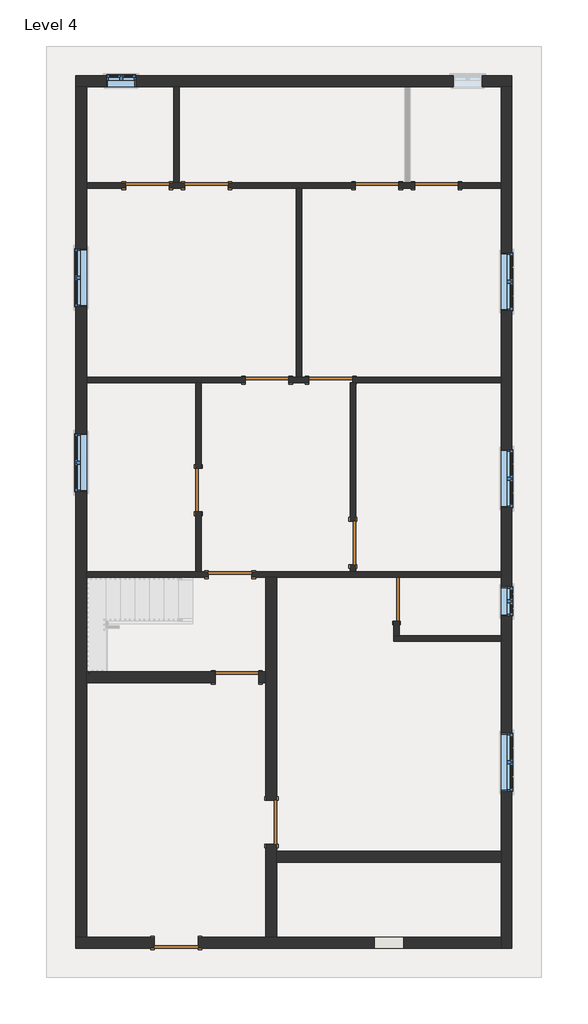
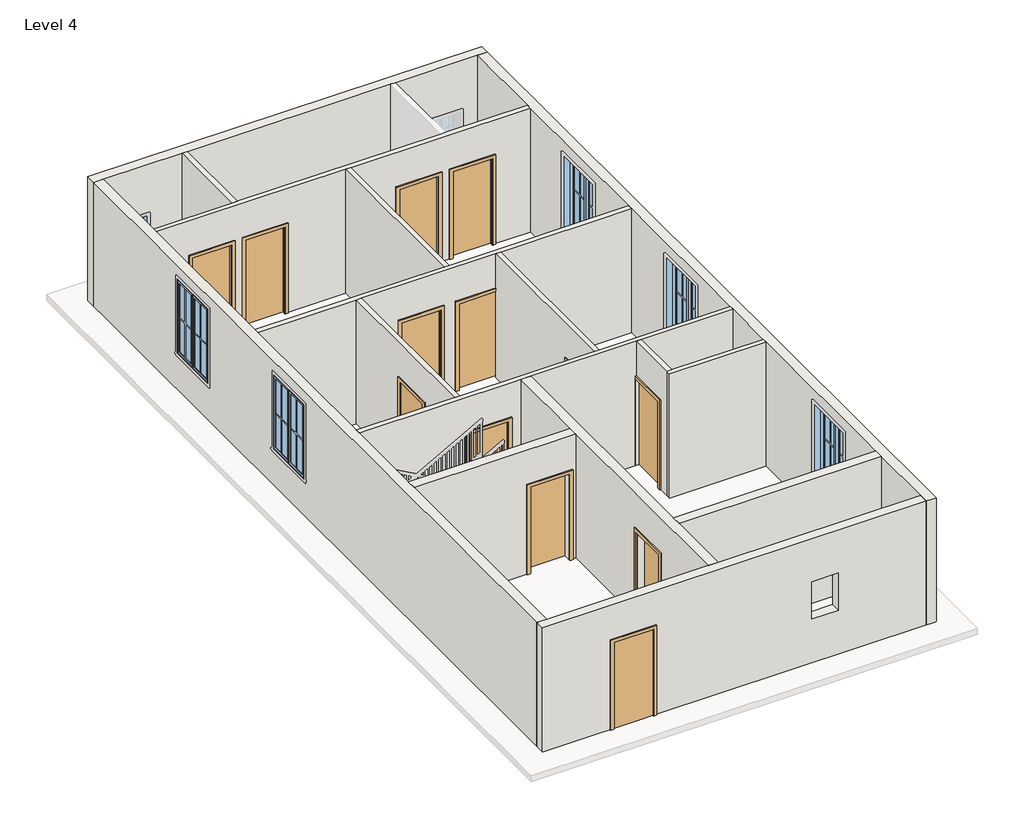
# One storey, part 1 of 3: 16 walls, 13 doors, 7 windows.
"""IFC4 building model written with IfcOpenShell, lengths in millimetres."""

from ifc_helpers import new_model, si_unit, frame, origin, place, context, project, spatial, polyline, outline, extrude, faceted_brep, transform, mapped, element, save
from components import door_305aa2a5, door_e5f9f3c4, door_0ca8825f, window_c417fced, window_6ca1769e

model = new_model("IFC4")

# Units and contexts
model_context = context("Model", 3, world=origin())
ifc_project = project(units=[si_unit("LENGTHUNIT", "METRE", prefix="MILLI")], contexts=[model_context])

# Site, building, storey
site = spatial("IfcSite", under=ifc_project)
building = spatial("IfcBuilding", under=site)
storey = spatial("IfcBuildingStorey", under=building, Name="Level 4", Elevation=9144.0)

# Doors
placement = place(None, origin())
door_shape = door_305aa2a5(model_context)
element("IfcDoor", 1, ObjectType="Single-Flush : 36\" x 84\"", at=placement, inside=storey, context=model_context, shape_type="MappedRepresentation", body=[
    mapped(door_shape, transform((4013.2, 11918.95, 9144.0), x_axis=(-1.0, 0.0, 0.0), y_axis=(0.0, -1.0, 0.0), z_axis=(0.0, 0.0, 1.0))),
])
element("IfcDoor", 2, ObjectType="Single-Flush : 36\" x 84\"", at=placement, inside=storey, context=model_context, shape_type="MappedRepresentation", body=[
    mapped(door_shape, transform((8832.85, 11918.95, 9144.0), x_axis=(-1.0, 0.0, 0.0), y_axis=(0.0, -1.0, 0.0), z_axis=(0.0, 0.0, 1.0))),
])
element("IfcDoor", 3, ObjectType="Single-Flush : 36\" x 84\"", at=placement, inside=storey, context=model_context, shape_type="MappedRepresentation", body=[
    mapped(door_shape, transform((6616.7, 7842.25, 9144.0), x_axis=(-1.0, 0.0, 0.0), y_axis=(0.0, -1.0, 0.0), z_axis=(0.0, 0.0, 1.0))),
])
element("IfcDoor", 4, ObjectType="Single-Flush : 36\" x 84\"", at=placement, inside=storey, context=model_context, shape_type="MappedRepresentation", body=[
    mapped(door_shape, transform((3841.75, 5537.2, 9144.0), x_axis=(0.0, -1.0, 0.0), y_axis=(1.0, 0.0, 0.0), z_axis=(0.0, 0.0, 1.0))),
])
door_2_shape = door_e5f9f3c4(model_context)
element("IfcDoor", 5, ObjectType="Single-Flush : 36\" x 84\"", at=placement, inside=storey, context=model_context, shape_type="MappedRepresentation", body=[
    mapped(door_2_shape, transform((2774.95, 11918.95, 9144.0), x_axis=(1.0, 0.0, 0.0), y_axis=(0.0, 1.0, 0.0), z_axis=(0.0, 0.0, 1.0))),
])
element("IfcDoor", 6, ObjectType="Single-Flush : 36\" x 84\"", at=placement, inside=storey, context=model_context, shape_type="MappedRepresentation", body=[
    mapped(door_2_shape, transform((7588.25, 11918.95, 9144.0), x_axis=(1.0, 0.0, 0.0), y_axis=(0.0, 1.0, 0.0), z_axis=(0.0, 0.0, 1.0))),
])
element("IfcDoor", 7, ObjectType="Single-Flush : 36\" x 84\"", at=placement, inside=storey, context=model_context, shape_type="MappedRepresentation", body=[
    mapped(door_2_shape, transform((5283.2, 7842.25, 9144.0), x_axis=(1.0, 0.0, 0.0), y_axis=(0.0, 1.0, 0.0), z_axis=(0.0, 0.0, 1.0))),
])
element("IfcDoor", 8, ObjectType="Single-Flush : 36\" x 84\"", at=placement, inside=storey, context=model_context, shape_type="MappedRepresentation", body=[
    mapped(door_2_shape, transform((4508.5, 3765.55, 9144.0), x_axis=(1.0, 0.0, 0.0), y_axis=(0.0, 1.0, 0.0), z_axis=(0.0, 0.0, 1.0))),
])
element("IfcDoor", 9, ObjectType="Single-Flush : 36\" x 84\"", at=placement, inside=storey, context=model_context, shape_type="MappedRepresentation", body=[
    mapped(door_2_shape, transform((7080.25, 4432.3, 9144.0), x_axis=(0.0, -1.0, 0.0), y_axis=(1.0, 0.0, 0.0), z_axis=(0.0, 0.0, 1.0))),
])
element("IfcDoor", 10, ObjectType="Single-Flush : 36\" x 84\"", at=placement, inside=storey, context=model_context, shape_type="MappedRepresentation", body=[
    mapped(door_2_shape, transform((7994.65, 3251.2, 9144.0), x_axis=(0.0, -1.0, 0.0), y_axis=(1.0, 0.0, 0.0), z_axis=(0.0, 0.0, 1.0))),
])
door_3_shape = door_0ca8825f(model_context)
element("IfcDoor", 11, ObjectType="Single-Flush : 36\" x 84\"", at=placement, inside=storey, context=model_context, shape_type="MappedRepresentation", body=[
    mapped(door_3_shape, transform((4648.2, 1612.9, 9144.0), x_axis=(1.0, 0.0, 0.0), y_axis=(0.0, 1.0, 0.0), z_axis=(0.0, 0.0, 1.0))),
])
element("IfcDoor", 12, ObjectType="Single-Flush : 36\" x 84\"", at=placement, inside=storey, context=model_context, shape_type="MappedRepresentation", body=[
    mapped(door_3_shape, transform((5372.1, -1422.4, 9144.0), x_axis=(0.0, -1.0, 0.0), y_axis=(1.0, 0.0, 0.0), z_axis=(0.0, 0.0, 1.0))),
])
element("IfcDoor", 13, ObjectType="Single-Flush : 36\" x 84\"", at=placement, inside=storey, context=model_context, shape_type="MappedRepresentation", body=[
    mapped(door_3_shape, transform((3378.2, -3949.7, 9144.0), x_axis=(-1.0, 0.0, 0.0), y_axis=(0.0, -1.0, 0.0), z_axis=(0.0, 0.0, 1.0))),
])

# Walls
element("IfcWall", 14, ObjectType="Generic - 5\"", at=placement, inside=storey, context=model_context, shape_type="Brep", body=[
    faceted_brep([(8045.45, 11861.8, 9144.0), (8375.65, 11861.8, 9144.0), (8375.65, 11861.8, 11277.6), (9290.05, 11861.8, 11277.6), (9290.05, 11861.8, 9144.0), (10185.4, 11861.8, 9144.0), (10185.4, 11861.8, 12192.0), (6007.1, 11861.8, 12192.0), (5892.8, 11861.8, 12192.0), (1498.6, 11861.8, 12192.0), (1498.6, 11861.8, 9144.0), (2317.75, 11861.8, 9144.0), (2317.75, 11861.8, 11277.6), (3232.15, 11861.8, 11277.6), (3232.15, 11861.8, 9144.0), (3556.0, 11861.8, 9144.0), (3556.0, 11861.8, 11277.6), (4470.4, 11861.8, 11277.6), (4470.4, 11861.8, 9144.0), (5892.8, 11861.8, 9144.0), (6007.1, 11861.8, 9144.0), (7131.05, 11861.8, 9144.0), (7131.05, 11861.8, 11277.6), (8045.45, 11861.8, 11277.6), (8375.65, 11976.1, 11277.6), (8375.65, 11976.1, 9144.0), (8280.4, 11976.1, 9144.0), (8166.1, 11976.1, 9144.0), (8045.45, 11976.1, 9144.0), (8045.45, 11976.1, 11277.6), (7131.05, 11976.1, 11277.6), (7131.05, 11976.1, 9144.0), (4470.4, 11976.1, 9144.0), (4470.4, 11976.1, 11277.6), (3556.0, 11976.1, 11277.6), (3556.0, 11976.1, 9144.0), (3441.7, 11976.1, 9144.0), (3327.4, 11976.1, 9144.0), (3232.15, 11976.1, 9144.0), (3232.15, 11976.1, 11277.6), (2317.75, 11976.1, 11277.6), (2317.75, 11976.1, 9144.0), (1498.6, 11976.1, 9144.0), (1498.6, 11976.1, 12192.0), (3327.4, 11976.1, 12192.0), (3441.7, 11976.1, 12192.0), (8166.1, 11976.1, 12192.0), (8280.4, 11976.1, 12192.0), (10185.4, 11976.1, 12192.0), (10185.4, 11976.1, 9144.0), (9290.05, 11976.1, 9144.0), (9290.05, 11976.1, 11277.6)], [[[0, 1, 2, 3, 4, 5, 6, 7, 8, 9, 10, 11, 12, 13, 14, 15, 16, 17, 18, 19, 20, 21, 22, 23]], [[24, 25, 26, 27, 28, 29, 30, 31, 32, 33, 34, 35, 36, 37, 38, 39, 40, 41, 42, 43, 44, 45, 46, 47, 48, 49, 50, 51]], [[11, 10, 42, 41]], [[15, 14, 38, 37, 36, 35]], [[21, 20, 19, 18, 32, 31]], [[50, 49, 5, 4]], [[28, 27, 26, 25, 1, 0]], [[9, 8, 7, 6, 48, 47, 46, 45, 44, 43]], [[6, 5, 49, 48]], [[10, 9, 43, 42]], [[16, 15, 35, 34]], [[17, 16, 34, 33]], [[18, 17, 33, 32]], [[39, 38, 14, 13]], [[40, 39, 13, 12]], [[41, 40, 12, 11]], [[29, 28, 0, 23]], [[30, 29, 23, 22]], [[31, 30, 22, 21]], [[2, 1, 25, 24]], [[3, 2, 24, 51]], [[4, 3, 51, 50]]]),
])
element("IfcWall", 15, ObjectType="Generic - 5\"", at=placement, inside=storey, context=model_context, shape_type="Brep", body=[
    faceted_brep([(5740.4, 7785.1, 9144.0), (6159.5, 7785.1, 9144.0), (6159.5, 7785.1, 11277.6), (7073.9, 7785.1, 11277.6), (7073.9, 7785.1, 9144.0), (7137.4, 7785.1, 9144.0), (10185.4, 7785.1, 9144.0), (10185.4, 7785.1, 12192.0), (7137.4, 7785.1, 12192.0), (7023.1, 7785.1, 12192.0), (3898.9, 7785.1, 12192.0), (3784.6, 7785.1, 12192.0), (1498.6, 7785.1, 12192.0), (1498.6, 7785.1, 9144.0), (3784.6, 7785.1, 9144.0), (3898.9, 7785.1, 9144.0), (4826.0, 7785.1, 9144.0), (4826.0, 7785.1, 11277.6), (5740.4, 7785.1, 11277.6), (6159.5, 7899.4, 11277.6), (6159.5, 7899.4, 9144.0), (6007.1, 7899.4, 9144.0), (5892.8, 7899.4, 9144.0), (5740.4, 7899.4, 9144.0), (5740.4, 7899.4, 11277.6), (4826.0, 7899.4, 11277.6), (4826.0, 7899.4, 9144.0), (1498.6, 7899.4, 9144.0), (1498.6, 7899.4, 12192.0), (5892.8, 7899.4, 12192.0), (6007.1, 7899.4, 12192.0), (10185.4, 7899.4, 12192.0), (10185.4, 7899.4, 9144.0), (7073.9, 7899.4, 9144.0), (7073.9, 7899.4, 11277.6)], [[[0, 1, 2, 3, 4, 5, 6, 7, 8, 9, 10, 11, 12, 13, 14, 15, 16, 17, 18]], [[19, 20, 21, 22, 23, 24, 25, 26, 27, 28, 29, 30, 31, 32, 33, 34]], [[16, 15, 14, 13, 27, 26]], [[33, 32, 6, 5, 4]], [[23, 22, 21, 20, 1, 0]], [[12, 11, 10, 9, 8, 7, 31, 30, 29, 28]], [[7, 6, 32, 31]], [[13, 12, 28, 27]], [[24, 23, 0, 18]], [[25, 24, 18, 17]], [[26, 25, 17, 16]], [[2, 1, 20, 19]], [[3, 2, 19, 34]], [[4, 3, 34, 33]]]),
])
element("IfcWall", 16, ObjectType="Generic - 5\"", at=placement, inside=storey, context=model_context, shape_type="SweptSolid", body=[
    extrude(outline(polyline([(5080.0, 11277.6), (5080.0, 9144.0), (3822.7, 9144.0), (3822.7, 12192.0), (7785.1, 12192.0), (7785.1, 9144.0), (5994.4, 9144.0), (5994.4, 11277.6), (5080.0, 11277.6)])), frame((3784.6, 0.0, 0.0), z_axis=(1.0, 0.0, 0.0), x_axis=(0.0, 1.0, 0.0)), (0.0, 0.0, 1.0), 114.3),
])
element("IfcWall", 17, ObjectType="Generic - 5\"", at=placement, inside=storey, context=model_context, shape_type="Brep", body=[
    faceted_brep([(4965.7, 3708.4, 11277.6), (4965.7, 3708.4, 9144.0), (5257.8, 3708.4, 9144.0), (5486.4, 3708.4, 9144.0), (10185.4, 3708.4, 9144.0), (10185.4, 3708.4, 12192.0), (8051.8, 3708.4, 12192.0), (7937.5, 3708.4, 12192.0), (5486.4, 3708.4, 12192.0), (5257.8, 3708.4, 12192.0), (1498.6, 3708.4, 12192.0), (1498.6, 3708.4, 9144.0), (4051.3, 3708.4, 9144.0), (4051.3, 3708.4, 11277.6), (10185.4, 3822.7, 9144.0), (7137.4, 3822.7, 9144.0), (7023.1, 3822.7, 9144.0), (4965.7, 3822.7, 9144.0), (4965.7, 3822.7, 11277.6), (4051.3, 3822.7, 11277.6), (4051.3, 3822.7, 9144.0), (3898.9, 3822.7, 9144.0), (3784.6, 3822.7, 9144.0), (1498.6, 3822.7, 9144.0), (1498.6, 3822.7, 12192.0), (3784.6, 3822.7, 12192.0), (3898.9, 3822.7, 12192.0), (7023.1, 3822.7, 12192.0), (7137.4, 3822.7, 12192.0), (10185.4, 3822.7, 12192.0)], [[[0, 1, 2, 3, 4, 5, 6, 7, 8, 9, 10, 11, 12, 13]], [[14, 15, 16, 17, 18, 19, 20, 21, 22, 23, 24, 25, 26, 27, 28, 29]], [[12, 11, 23, 22, 21, 20]], [[4, 3, 2, 1, 17, 16, 15, 14]], [[10, 9, 8, 7, 6, 5, 29, 28, 27, 26, 25, 24]], [[5, 4, 14, 29]], [[11, 10, 24, 23]], [[18, 17, 1, 0]], [[19, 18, 0, 13]], [[20, 19, 13, 12]]]),
])
element("IfcWall", 18, ObjectType="Generic - 5\"", at=placement, inside=storey, context=model_context, shape_type="Brep", body=[
    faceted_brep([(10185.4, 2489.2, 9144.0), (8051.8, 2489.2, 9144.0), (7937.5, 2489.2, 9144.0), (7937.5, 2489.2, 12192.0), (8051.8, 2489.2, 12192.0), (10185.4, 2489.2, 12192.0), (10185.4, 2374.9, 9144.0), (10185.4, 2374.9, 12192.0), (7937.5, 2374.9, 12192.0), (7937.5, 2374.9, 9144.0)], [[[0, 1, 2, 3, 4, 5]], [[6, 7, 8, 9]], [[2, 1, 0, 6, 9]], [[5, 4, 3, 8, 7]], [[0, 5, 7, 6]], [[3, 2, 9, 8]]]),
])
element("IfcWall", 19, ObjectType="Generic - 5\"", at=placement, inside=storey, context=model_context, shape_type="SweptSolid", body=[
    extrude(outline(polyline([(2489.2, 12192.0), (3708.4, 12192.0), (3708.4, 11277.6), (2794.0, 11277.6), (2794.0, 9144.0), (2489.2, 9144.0), (2489.2, 12192.0)])), frame((7937.5, 0.0, 0.0), z_axis=(1.0, 0.0, 0.0), x_axis=(0.0, 1.0, 0.0)), (0.0, 0.0, 1.0), 114.3),
])
element("IfcWall", 20, ObjectType="Generic - 5\"", at=placement, inside=storey, context=model_context, shape_type="Brep", body=[
    faceted_brep([(7023.1, 3975.1, 11277.6), (7023.1, 3975.1, 9144.0), (7023.1, 3822.7, 9144.0), (7023.1, 3822.7, 12192.0), (7023.1, 7785.1, 12192.0), (7023.1, 7785.1, 9144.0), (7023.1, 4889.5, 9144.0), (7023.1, 4889.5, 11277.6), (7137.4, 3822.7, 9144.0), (7137.4, 3975.1, 9144.0), (7137.4, 3975.1, 11277.6), (7137.4, 4889.5, 11277.6), (7137.4, 4889.5, 9144.0), (7137.4, 7785.1, 9144.0), (7137.4, 7785.1, 12192.0), (7137.4, 3822.7, 12192.0), (7073.9, 7785.1, 9144.0)], [[[0, 1, 2, 3, 4, 5, 6, 7]], [[8, 9, 10, 11, 12, 13, 14, 15]], [[6, 5, 16, 13, 12]], [[2, 1, 9, 8]], [[4, 3, 15, 14]], [[5, 4, 14, 13, 16]], [[3, 2, 8, 15]], [[10, 9, 1, 0]], [[11, 10, 0, 7]], [[12, 11, 7, 6]]]),
])
element("IfcWall", 21, ObjectType="Generic - 5\"", at=placement, inside=storey, context=model_context, shape_type="SweptSolid", body=[
    extrude(outline(polyline([(3327.4, 11976.1), (3327.4, 13995.4), (3441.7, 13995.4), (3441.7, 11976.1), (3327.4, 11976.1)])), frame((0.0, 0.0, 9144.0), z_axis=(0.0, 0.0, 1.0), x_axis=(1.0, 0.0, 0.0)), (0.0, 0.0, 1.0), 3048.0),
])
element("IfcWall", 22, ObjectType="Generic - 5\"", at=placement, inside=storey, context=model_context, shape_type="SweptSolid", body=[
    extrude(outline(polyline([(5892.8, 7899.4), (5892.8, 11861.8), (6007.1, 11861.8), (6007.1, 7899.4), (5892.8, 7899.4)])), frame((0.0, 0.0, 9144.0), z_axis=(0.0, 0.0, 1.0), x_axis=(1.0, 0.0, 0.0)), (0.0, 0.0, 1.0), 3048.0),
])
element("IfcWall", 23, ObjectType="Generic - 8\"", at=placement, inside=storey, context=model_context, shape_type="Brep", body=[
    faceted_brep([(1270.0, 13995.4, 9144.0), (1498.6, 13995.4, 9144.0), (3327.4, 13995.4, 9144.0), (3441.7, 13995.4, 9144.0), (8166.1, 13995.4, 9144.0), (8280.4, 13995.4, 9144.0), (10185.4, 13995.4, 9144.0), (10414.0, 13995.4, 9144.0), (10414.0, 13995.4, 12192.0), (10185.4, 13995.4, 12192.0), (8280.4, 13995.4, 12192.0), (8166.1, 13995.4, 12192.0), (3441.7, 13995.4, 12192.0), (3327.4, 13995.4, 12192.0), (1498.6, 13995.4, 12192.0), (1270.0, 13995.4, 12192.0), (9791.7, 13995.4, 10972.8), (9791.7, 13995.4, 10058.4), (9182.1, 13995.4, 10058.4), (9182.1, 13995.4, 10972.8), (2527.3, 13995.4, 10972.8), (2527.3, 13995.4, 10058.4), (1917.7, 13995.4, 10058.4), (1917.7, 13995.4, 10972.8), (1270.0, 14224.0, 9144.0), (1270.0, 14224.0, 12192.0), (10414.0, 14224.0, 12192.0), (10414.0, 14224.0, 9144.0), (9791.7, 14224.0, 10972.8), (9182.1, 14224.0, 10972.8), (9182.1, 14224.0, 10058.4), (9791.7, 14224.0, 10058.4), (2527.3, 14224.0, 10972.8), (1917.7, 14224.0, 10972.8), (1917.7, 14224.0, 10058.4), (2527.3, 14224.0, 10058.4)], [[[0, 1, 2, 3, 4, 5, 6, 7, 8, 9, 10, 11, 12, 13, 14, 15], [16, 17, 18, 19], [20, 21, 22, 23]], [[24, 25, 26, 27], [28, 29, 30, 31], [32, 33, 34, 35]], [[7, 6, 5, 4, 3, 2, 1, 0, 24, 27]], [[15, 14, 13, 12, 11, 10, 9, 8, 26, 25]], [[8, 7, 27, 26]], [[0, 15, 25, 24]], [[17, 16, 28, 31]], [[18, 17, 31, 30]], [[19, 18, 30, 29]], [[16, 19, 29, 28]], [[21, 20, 32, 35]], [[22, 21, 35, 34]], [[23, 22, 34, 33]], [[20, 23, 33, 32]]]),
])
element("IfcWall", 24, ObjectType="Generic - 8\"", at=placement, inside=storey, context=model_context, shape_type="Brep", body=[
    faceted_brep([(10185.4, 13995.4, 9144.0), (10185.4, 11976.1, 9144.0), (10185.4, 11861.8, 9144.0), (10185.4, 7899.4, 9144.0), (10185.4, 7785.1, 9144.0), (10185.4, 3822.7, 9144.0), (10185.4, 3708.4, 9144.0), (10185.4, 2489.2, 9144.0), (10185.4, 2374.9, 9144.0), (10185.4, -2032.0, 9144.0), (10185.4, -2260.6, 9144.0), (10185.4, -3835.4, 9144.0), (10185.4, -4064.0, 9144.0), (10185.4, -4064.0, 12192.0), (10185.4, -3835.4, 12192.0), (10185.4, -2260.6, 12192.0), (10185.4, -2032.0, 12192.0), (10185.4, 2374.9, 12192.0), (10185.4, 2489.2, 12192.0), (10185.4, 3708.4, 12192.0), (10185.4, 3822.7, 12192.0), (10185.4, 7785.1, 12192.0), (10185.4, 7899.4, 12192.0), (10185.4, 11861.8, 12192.0), (10185.4, 11976.1, 12192.0), (10185.4, 13995.4, 12192.0), (10185.4, 9296.4, 11887.2), (10185.4, 9296.4, 10058.4), (10185.4, 10515.6, 10058.4), (10185.4, 10515.6, 11887.2), (10185.4, 5168.9, 11887.2), (10185.4, 5168.9, 10058.4), (10185.4, 6388.1, 10058.4), (10185.4, 6388.1, 11887.2), (10185.4, -774.7, 11887.2), (10185.4, -774.7, 10058.4), (10185.4, 444.5, 10058.4), (10185.4, 444.5, 11887.2), (10185.4, 2901.95, 10972.8), (10185.4, 2901.95, 10058.4), (10185.4, 3511.55, 10058.4), (10185.4, 3511.55, 10972.8), (10414.0, 13995.4, 9144.0), (10414.0, 13995.4, 12192.0), (10414.0, -4064.0, 12192.0), (10414.0, -4064.0, 9144.0), (10414.0, 9296.4, 11887.2), (10414.0, 10515.6, 11887.2), (10414.0, 10515.6, 10058.4), (10414.0, 9296.4, 10058.4), (10414.0, 5168.9, 11887.2), (10414.0, 6388.1, 11887.2), (10414.0, 6388.1, 10058.4), (10414.0, 5168.9, 10058.4), (10414.0, -774.7, 11887.2), (10414.0, 444.5, 11887.2), (10414.0, 444.5, 10058.4), (10414.0, -774.7, 10058.4), (10414.0, 2901.95, 10972.8), (10414.0, 3511.55, 10972.8), (10414.0, 3511.55, 10058.4), (10414.0, 2901.95, 10058.4)], [[[0, 1, 2, 3, 4, 5, 6, 7, 8, 9, 10, 11, 12, 13, 14, 15, 16, 17, 18, 19, 20, 21, 22, 23, 24, 25], [26, 27, 28, 29], [30, 31, 32, 33], [34, 35, 36, 37], [38, 39, 40, 41]], [[42, 43, 44, 45], [46, 47, 48, 49], [50, 51, 52, 53], [54, 55, 56, 57], [58, 59, 60, 61]], [[12, 11, 10, 9, 8, 7, 6, 5, 4, 3, 2, 1, 0, 42, 45]], [[25, 24, 23, 22, 21, 20, 19, 18, 17, 16, 15, 14, 13, 44, 43]], [[0, 25, 43, 42]], [[13, 12, 45, 44]], [[27, 26, 46, 49]], [[28, 27, 49, 48]], [[29, 28, 48, 47]], [[26, 29, 47, 46]], [[31, 30, 50, 53]], [[32, 31, 53, 52]], [[33, 32, 52, 51]], [[30, 33, 51, 50]], [[35, 34, 54, 57]], [[36, 35, 57, 56]], [[37, 36, 56, 55]], [[34, 37, 55, 54]], [[39, 38, 58, 61]], [[40, 39, 61, 60]], [[41, 40, 60, 59]], [[38, 41, 59, 58]]]),
])
element("IfcWall", 25, ObjectType="Generic - 8\"", at=placement, inside=storey, context=model_context, shape_type="Brep", body=[
    faceted_brep([(2921.0, -3835.4, 11277.6), (2921.0, -3835.4, 9144.0), (1498.6, -3835.4, 9144.0), (1270.0, -3835.4, 9144.0), (1270.0, -3835.4, 12192.0), (1498.6, -3835.4, 12192.0), (5257.8, -3835.4, 12192.0), (5486.4, -3835.4, 12192.0), (10185.4, -3835.4, 12192.0), (10185.4, -3835.4, 9144.0), (5486.4, -3835.4, 9144.0), (5257.8, -3835.4, 9144.0), (3835.4, -3835.4, 9144.0), (3835.4, -3835.4, 11277.6), (7531.1, -3835.4, 11139.4873604), (7531.1, -3835.4, 10225.0873604), (8140.7, -3835.4, 10225.0873604), (8140.7, -3835.4, 11139.4873604), (1270.0, -4064.0, 9144.0), (2921.0, -4064.0, 9144.0), (2921.0, -4064.0, 11277.6), (3835.4, -4064.0, 11277.6), (3835.4, -4064.0, 9144.0), (10185.4, -4064.0, 9144.0), (10185.4, -4064.0, 12192.0), (1270.0, -4064.0, 12192.0), (7531.1, -4064.0, 11139.4873604), (8140.7, -4064.0, 11139.4873604), (8140.7, -4064.0, 10225.0873604), (7531.1, -4064.0, 10225.0873604)], [[[0, 1, 2, 3, 4, 5, 6, 7, 8, 9, 10, 11, 12, 13], [14, 15, 16, 17]], [[18, 19, 20, 21, 22, 23, 24, 25], [26, 27, 28, 29]], [[3, 2, 1, 19, 18]], [[12, 11, 10, 9, 23, 22]], [[8, 7, 6, 5, 4, 25, 24]], [[9, 8, 24, 23]], [[4, 3, 18, 25]], [[20, 19, 1, 0]], [[21, 20, 0, 13]], [[22, 21, 13, 12]], [[15, 14, 26, 29]], [[16, 15, 29, 28]], [[17, 16, 28, 27]], [[14, 17, 27, 26]]]),
])
element("IfcWall", 26, ObjectType="Generic - 8\"", at=placement, inside=storey, context=model_context, shape_type="Brep", body=[
    faceted_brep([(1498.6, -3835.4, 9144.0), (1498.6, 1498.6, 9144.0), (1498.6, 1727.2, 9144.0), (1498.6, 3708.4, 9144.0), (1498.6, 3822.7, 9144.0), (1498.6, 7785.1, 9144.0), (1498.6, 7899.4, 9144.0), (1498.6, 11861.8, 9144.0), (1498.6, 11976.1, 9144.0), (1498.6, 13995.4, 9144.0), (1498.6, 13995.4, 12192.0), (1498.6, 11976.1, 12192.0), (1498.6, 11861.8, 12192.0), (1498.6, 7899.4, 12192.0), (1498.6, 7785.1, 12192.0), (1498.6, 3822.7, 12192.0), (1498.6, 3708.4, 12192.0), (1498.6, 1727.2, 12192.0), (1498.6, 1498.6, 12192.0), (1498.6, -3835.4, 12192.0), (1498.6, 6724.65, 11887.2), (1498.6, 6724.65, 10058.4), (1498.6, 5505.45, 10058.4), (1498.6, 5505.45, 11887.2), (1498.6, 10598.15, 11887.2), (1498.6, 10598.15, 10058.4), (1498.6, 9378.95, 10058.4), (1498.6, 9378.95, 11887.2), (1270.0, -3835.4, 9144.0), (1270.0, -3835.4, 12192.0), (1270.0, 13995.4, 12192.0), (1270.0, 13995.4, 9144.0), (1270.0, 6724.65, 11887.2), (1270.0, 5505.45, 11887.2), (1270.0, 5505.45, 10058.4), (1270.0, 6724.65, 10058.4), (1270.0, 10598.15, 11887.2), (1270.0, 9378.95, 11887.2), (1270.0, 9378.95, 10058.4), (1270.0, 10598.15, 10058.4)], [[[0, 1, 2, 3, 4, 5, 6, 7, 8, 9, 10, 11, 12, 13, 14, 15, 16, 17, 18, 19], [20, 21, 22, 23], [24, 25, 26, 27]], [[28, 29, 30, 31], [32, 33, 34, 35], [36, 37, 38, 39]], [[9, 8, 7, 6, 5, 4, 3, 2, 1, 0, 28, 31]], [[19, 18, 17, 16, 15, 14, 13, 12, 11, 10, 30, 29]], [[10, 9, 31, 30]], [[0, 19, 29, 28]], [[21, 20, 32, 35]], [[22, 21, 35, 34]], [[23, 22, 34, 33]], [[20, 23, 33, 32]], [[25, 24, 36, 39]], [[26, 25, 39, 38]], [[27, 26, 38, 37]], [[24, 27, 37, 36]]]),
])
element("IfcWall", 27, ObjectType="Generic - 8\"", at=placement, inside=storey, context=model_context, shape_type="SweptSolid", body=[
    extrude(outline(polyline([(11277.6, 5105.4), (9144.0, 5105.4), (9144.0, 5257.8), (12192.0, 5257.8), (12192.0, 1498.6), (9144.0, 1498.6), (9144.0, 4191.0), (11277.6, 4191.0), (11277.6, 5105.4)])), frame((0.0, 1498.6, 0.0), z_axis=(0.0, 1.0, 0.0), x_axis=(0.0, 0.0, 1.0)), (0.0, 0.0, 1.0), 228.6),
])
element("IfcWall", 28, ObjectType="Generic - 8\"", at=placement, inside=storey, context=model_context, shape_type="Brep", body=[
    faceted_brep([(5257.8, -1879.6, 11277.6), (5257.8, -1879.6, 9144.0), (5257.8, -3835.4, 9144.0), (5257.8, -3835.4, 12192.0), (5257.8, 1498.6, 12192.0), (5257.8, 1727.2, 12192.0), (5257.8, 3708.4, 12192.0), (5257.8, 3708.4, 9144.0), (5257.8, 1727.2, 9144.0), (5257.8, 1498.6, 9144.0), (5257.8, -965.2, 9144.0), (5257.8, -965.2, 11277.6), (5486.4, -3835.4, 9144.0), (5486.4, -2260.6, 9144.0), (5486.4, -2032.0, 9144.0), (5486.4, -1879.6, 9144.0), (5486.4, -1879.6, 11277.6), (5486.4, -965.2, 11277.6), (5486.4, -965.2, 9144.0), (5486.4, 3708.4, 9144.0), (5486.4, 3708.4, 12192.0), (5486.4, -2032.0, 12192.0), (5486.4, -2260.6, 12192.0), (5486.4, -3835.4, 12192.0)], [[[0, 1, 2, 3, 4, 5, 6, 7, 8, 9, 10, 11]], [[12, 13, 14, 15, 16, 17, 18, 19, 20, 21, 22, 23]], [[2, 1, 15, 14, 13, 12]], [[10, 9, 8, 7, 19, 18]], [[6, 5, 4, 3, 23, 22, 21, 20]], [[3, 2, 12, 23]], [[7, 6, 20, 19]], [[16, 15, 1, 0]], [[17, 16, 0, 11]], [[18, 17, 11, 10]]]),
])
element("IfcWall", 29, ObjectType="Generic - 8\"", at=placement, inside=storey, context=model_context, shape_type="SweptSolid", body=[
    extrude(outline(polyline([(10185.4, -2260.6), (5486.4, -2260.6), (5486.4, -2032.0), (10185.4, -2032.0), (10185.4, -2260.6)])), frame((0.0, 0.0, 9144.0), z_axis=(0.0, 0.0, 1.0), x_axis=(1.0, 0.0, 0.0)), (0.0, 0.0, 1.0), 3048.0),
])

# Windows
window_shape = window_c417fced(model_context)
element("IfcWindow", 30, ObjectType="Window-Casement-Double : 24\" x 36\"", at=placement, inside=storey, context=model_context, shape_type="MappedRepresentation", body=[
    mapped(window_shape, transform((10299.7, 3206.75, 9144.0), x_axis=(0.0, -1.0, 0.0), y_axis=(1.0, 0.0, 0.0), z_axis=(0.0, 0.0, 1.0))),
])
element("IfcWindow", 31, ObjectType="Window-Casement-Double : 24\" x 36\"", at=placement, inside=storey, context=model_context, shape_type="MappedRepresentation", body=[
    mapped(window_shape, transform((2222.5, 14109.7, 9144.0), x_axis=(1.0, 0.0, 0.0), y_axis=(0.0, 1.0, 0.0), z_axis=(0.0, 0.0, 1.0))),
])
window_2_shape = window_6ca1769e(model_context)
element("IfcWindow", 32, ObjectType="Window-Casement-Double : 48\" x 72\"", at=placement, inside=storey, context=model_context, shape_type="MappedRepresentation", body=[
    mapped(window_2_shape, transform((1384.3, 6115.05, 9144.0), x_axis=(0.0, 1.0, 0.0), y_axis=(-1.0, 0.0, 0.0), z_axis=(0.0, 0.0, 1.0))),
])
element("IfcWindow", 33, ObjectType="Window-Casement-Double : 48\" x 72\"", at=placement, inside=storey, context=model_context, shape_type="MappedRepresentation", body=[
    mapped(window_2_shape, transform((1384.3, 9988.55, 9144.0), x_axis=(0.0, 1.0, 0.0), y_axis=(-1.0, 0.0, 0.0), z_axis=(0.0, 0.0, 1.0))),
])
element("IfcWindow", 34, ObjectType="Window-Casement-Double : 48\" x 72\"", at=placement, inside=storey, context=model_context, shape_type="MappedRepresentation", body=[
    mapped(window_2_shape, transform((10299.7, 9906.0, 9144.0), x_axis=(0.0, -1.0, 0.0), y_axis=(1.0, 0.0, 0.0), z_axis=(0.0, 0.0, 1.0))),
])
element("IfcWindow", 35, ObjectType="Window-Casement-Double : 48\" x 72\"", at=placement, inside=storey, context=model_context, shape_type="MappedRepresentation", body=[
    mapped(window_2_shape, transform((10299.7, 5778.5, 9144.0), x_axis=(0.0, -1.0, 0.0), y_axis=(1.0, 0.0, 0.0), z_axis=(0.0, 0.0, 1.0))),
])
element("IfcWindow", 36, ObjectType="Window-Casement-Double : 48\" x 72\"", at=placement, inside=storey, context=model_context, shape_type="MappedRepresentation", body=[
    mapped(window_2_shape, transform((10299.7, -165.1, 9144.0), x_axis=(0.0, -1.0, 0.0), y_axis=(1.0, 0.0, 0.0), z_axis=(0.0, 0.0, 1.0))),
])

save(model, "model.ifc")

# Revit data of these elements
# Type "Single-Flush : 36\" x 84\""
#   Type Mark = "1"
#   Construction Type Id = "MDOOR"
#   Assembly Code = "C1020"
#   Analytic Construction = "Metal"
#   Thickness = 0' - 2"
#   Heat Transfer Coefficient (U) = 0.651978 BTU/(h·ft²·°F)
#   Height = 7' - 0"
#   Trim Projection Ext = 0' - 1"
#   Trim Projection Int = 0' - 1"
#   Trim Width = 0' - 3"
#   Width = 3' - 0"
#   Define Thermal Properties by = 1
#   Define Thermal Properties by = 1
#   Door Material = Door - Panel
#   Frame Material = Door - Frame
#   Visual Light Transmittance = 0
#   Solar Heat Gain Coefficient = 0
#   Function = (empty or 0)
#   Wall Closure = (empty or 0)
# Type "Generic - 5\""
#   Assembly Code = "B2010"
#   Layers, outside or top first: 0' - 4 1/2" no material (function 1)
# Type "Generic - 8\""
#   Assembly Code = "B2010"
#   Layers, outside or top first: 0' - 9" "Parking Stripe" (function 1)
# Type "Window-Casement-Double : 24\" x 36\""
#   Type Mark = "14"
#   Fire Rating = "0.5h"
#   Assembly Code = "B2020100"
#   Analytic Construction = "Double glazing - domestic"
#   Frame Extension [instance default] = 0' - 0 1/4"
#   Window Inset [instance default] = 0' - 0"
#   Wall Thickness [instance default] = 0' - 6"
#   Interior Wall Closure [instance default] = 0' - 2 1/4"
#   Half Width = 1' - 0"
#   Visual Light Transmittance = 0.81
#   Thermal Resistance (R) = 1.8146 (h·ft²·°F)/BTU
#   Solar Heat Gain Coefficient = 0.76
#   Rough Width = 2' - 0 1/2"
#   Rough Height = 3' - 0 1/2"
#   Height = 3' - 0"
#   Heat Transfer Coefficient (U) = 0.5511 BTU/(h·ft²·°F)
#   Exterior Wall Closure [instance default] = 0' - 1 1/4"
#   Extension Jamb [instance default] = 0' - 2 1/4"
#   Default Sill Height = 3' - 0"
#   Width = 2' - 0"
#   Define Thermal Properties by = 0
#   Muntin Visibility = yes
#   Interior Trim Visibility [instance default] = yes
#   Exterior Trim Visibility [instance default] = yes
#   Extension Jamb Visibility [instance default] = yes
#   Interior Trim Material = Wood - Stained
#   Muntin Pattern = Muntin Pattern_2x2 : Muntin Pattern_2x2
#   Interior Trim = Trim-Window-Interior-Flat : Picture Frame
#   Interior Frame Material = Wood - Stained
#   Glass Panel Material = Glass
#   Exterior Trim Material = Clad - White
#   Exterior Trim = Trim-Window-Exterior-Flat : with Sill
#   Exterior Frame Material = Clad - White
#   Wall Closure = (empty or 0)
# Type "Window-Casement-Double : 48\" x 72\""
#   Type Mark = "17"
#   Fire Rating = "0.5h"
#   Assembly Code = "B2020100"
#   Analytic Construction = "Double glazing - domestic"
#   Frame Extension [instance default] = 0' - 0 1/4"
#   Window Inset [instance default] = 0' - 0"
#   Wall Thickness [instance default] = 0' - 6"
#   Interior Wall Closure [instance default] = 0' - 2 1/4"
#   Half Width = 2' - 0"
#   Visual Light Transmittance = 0.81
#   Thermal Resistance (R) = 1.8146 (h·ft²·°F)/BTU
#   Solar Heat Gain Coefficient = 0.76
#   Rough Width = 4' - 0 1/2"
#   Rough Height = 6' - 0 1/2"
#   Height = 6' - 0"
#   Heat Transfer Coefficient (U) = 0.5511 BTU/(h·ft²·°F)
#   Exterior Wall Closure [instance default] = 0' - 1 1/4"
#   Extension Jamb [instance default] = 0' - 2 1/4"
#   Default Sill Height = 3' - 0"
#   Width = 4' - 0"
#   Define Thermal Properties by = 0
#   Muntin Visibility = yes
#   Interior Trim Visibility [instance default] = yes
#   Exterior Trim Visibility [instance default] = yes
#   Extension Jamb Visibility [instance default] = yes
#   Interior Trim Material = Wood - Stained
#   Muntin Pattern = Muntin Pattern_2x2 : Muntin Pattern_2x2
#   Interior Trim = Trim-Window-Interior-Flat : Picture Frame
#   Interior Frame Material = Wood - Stained
#   Glass Panel Material = Glass
#   Exterior Trim Material = Clad - White
#   Exterior Trim = Trim-Window-Exterior-Flat : with Sill
#   Exterior Frame Material = Clad - White
#   Wall Closure = (empty or 0)
# Elements 1, 2, 3, 4, 5, 6, 7, 8, 9, 10, 11, 12, 13 (IfcDoor, "Single-Flush : 36\" x 84\"")
#   Phase Created = New Construction
#   Materials on its faces: "Door - Frame", "Door - Panel"
# Elements 14, 15, 16, 17, 18, 19, 20, 21, 22 (IfcWall, "Generic - 5\"")
#   Top Offset = 0' - 0"
#   Base Offset = 0' - 0"
#   wall height = 10' - 0"
#   Phase Created = New Construction
#   Base Constraint = Level 4
#   Top Constraint = Level 5
#   Materials on its faces: "Default Wall"
# Elements 23, 24, 25, 26, 27, 28, 29 (IfcWall, "Generic - 8\"")
#   Top Offset = 0' - 0"
#   Base Offset = 0' - 0"
#   Unconnected Height = 10' - 0"
#   wall height = 10' - 0"
#   Phase Created = New Construction
#   Base Constraint = Level 4
#   Materials on its faces: "Parking Stripe"
# Element 30 (IfcWindow, "Window-Casement-Double : 24\" x 36\"")
#   Mark = "30"
#   Window Inset = 0' - 0"
#   Interior Wall Closure = 0' - 2 1/4"
#   Frame Extension = 0' - 0 1/4"
#   Exterior Wall Closure = 0' - 1 1/4"
#   Interior Trim Visibility = yes
#   Exterior Trim Visibility = yes
#   Phase Created = New Construction
#   Materials on its faces: "Wood - Stained", "Glass", "Clad - White"
# Element 31 (IfcWindow, "Window-Casement-Double : 24\" x 36\"")
#   Mark = "32"
#   Window Inset = 0' - 0"
#   Interior Wall Closure = 0' - 2 1/4"
#   Frame Extension = 0' - 0 1/4"
#   Exterior Wall Closure = 0' - 1 1/4"
#   Interior Trim Visibility = yes
#   Exterior Trim Visibility = yes
#   Phase Created = New Construction
#   Materials on its faces: "Wood - Stained", "Glass", "Clad - White"
# Element 32 (IfcWindow, "Window-Casement-Double : 48\" x 72\"")
#   Mark = "25"
#   Window Inset = 0' - 0"
#   Interior Wall Closure = 0' - 2 1/4"
#   Frame Extension = 0' - 0 1/4"
#   Exterior Wall Closure = 0' - 1 1/4"
#   Interior Trim Visibility = yes
#   Exterior Trim Visibility = yes
#   Phase Created = New Construction
#   Materials on its faces: "Wood - Stained", "Glass", "Clad - White"
# Element 33 (IfcWindow, "Window-Casement-Double : 48\" x 72\"")
#   Mark = "26"
#   Window Inset = 0' - 0"
#   Interior Wall Closure = 0' - 2 1/4"
#   Frame Extension = 0' - 0 1/4"
#   Exterior Wall Closure = 0' - 1 1/4"
#   Interior Trim Visibility = yes
#   Exterior Trim Visibility = yes
#   Phase Created = New Construction
#   Materials on its faces: "Wood - Stained", "Glass", "Clad - White"
# Element 34 (IfcWindow, "Window-Casement-Double : 48\" x 72\"")
#   Mark = "27"
#   Window Inset = 0' - 0"
#   Interior Wall Closure = 0' - 2 1/4"
#   Frame Extension = 0' - 0 1/4"
#   Exterior Wall Closure = 0' - 1 1/4"
#   Interior Trim Visibility = yes
#   Exterior Trim Visibility = yes
#   Phase Created = New Construction
#   Materials on its faces: "Wood - Stained", "Glass", "Clad - White"
# Element 35 (IfcWindow, "Window-Casement-Double : 48\" x 72\"")
#   Mark = "28"
#   Window Inset = 0' - 0"
#   Interior Wall Closure = 0' - 2 1/4"
#   Frame Extension = 0' - 0 1/4"
#   Exterior Wall Closure = 0' - 1 1/4"
#   Interior Trim Visibility = yes
#   Exterior Trim Visibility = yes
#   Phase Created = New Construction
#   Materials on its faces: "Wood - Stained", "Glass", "Clad - White"
# Element 36 (IfcWindow, "Window-Casement-Double : 48\" x 72\"")
#   Mark = "29"
#   Window Inset = 0' - 0"
#   Interior Wall Closure = 0' - 2 1/4"
#   Frame Extension = 0' - 0 1/4"
#   Exterior Wall Closure = 0' - 1 1/4"
#   Interior Trim Visibility = yes
#   Exterior Trim Visibility = yes
#   Phase Created = New Construction
#   Materials on its faces: "Wood - Stained", "Glass", "Clad - White"
# Materials
#   "Door - Panel": class "Wood", colour RGB 210 159 95, transparency 0, Cost = 0
#   "Door - Frame": colour RGB 118 70 51, transparency 0, Cost = 0
#   "Parking Stripe": class "Paint", colour RGB 250 250 91, transparency 0, Cost = 0
#   "Wood - Stained": class "Wood", colour RGB 224 178 126, transparency 0, Cost = 0
#   "Glass": class "Glass", colour RGB 0 128 192, transparency 0.75, Description = "Soda Lime Glass", Cost = 0
#   "Clad - White": class "Wood", colour RGB 242 242 238, transparency 0, Cost = 0
#   "Default Wall": colour RGB 128 128 128, transparency 0, Cost = 0
